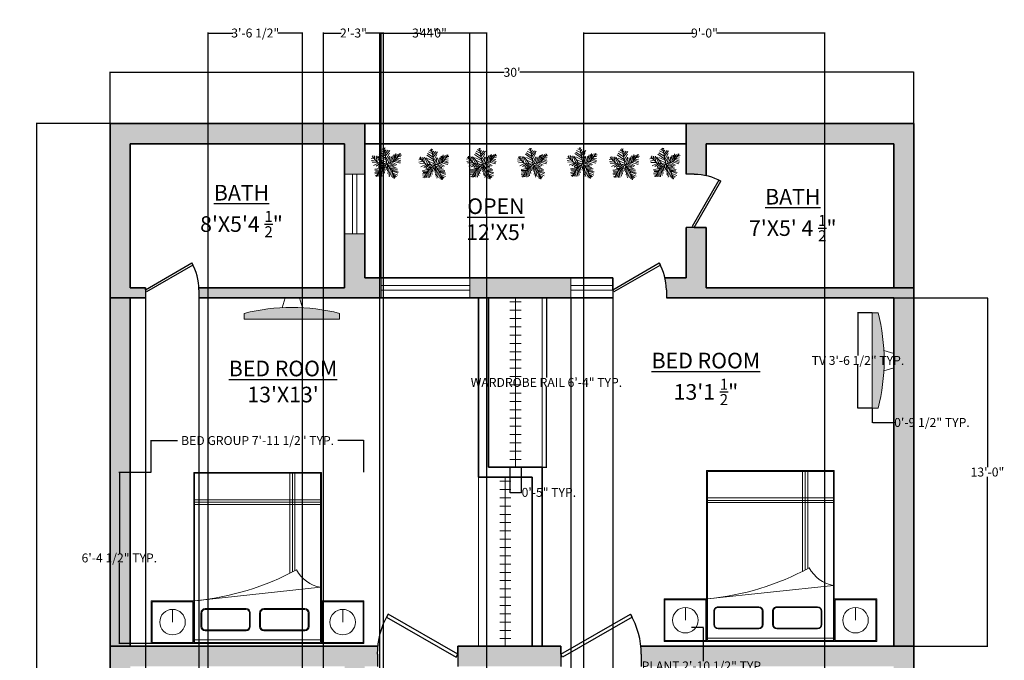
# Model space of a CAD drawing. Units: inches. Extents: x -37 to 408, y -619 to 75.
# Tile 4 of 4: x -37 to 404, y -212 to 75. Entities that reach past the tile are written whole.
import ezdxf

# ---------------------------------------------------------------- set-up
doc = ezdxf.new("R2010")
doc.units = ezdxf.units.IN
doc.header["$MEASUREMENT"] = 0
for name, color, linetype, lineweight in [('A-ANNO-DIMS', 2, 'Continuous', 18), ('A-AREA-IDEN', 7, 'Continuous', 25), ('A-DOOR', 4, 'Continuous', 25), ('A-EQPM', 9, 'Continuous', 18), ('A-FLOR-CASE', 8, 'Continuous', 18), ('A-FURN', 8, 'Continuous', 18), ('A-GLAZ', 4, 'Continuous', 18), ('A-WALL', 7, 'Continuous', 35), ('A-WALL-PATT', 16, 'Continuous', 13), ('tree', 3, 'Continuous', 13)]:
    doc.layers.add(name, color=color, linetype=linetype, lineweight=lineweight)
doc.styles.get("Standard").update_dxf_attribs({"font": 'arial.ttf'})
doc.dimstyles.get("Standard").update_dxf_attribs({"dimtxt": 4, "dimasz": 0.18, "dimexe": 0.18, "dimexo": 0.0625, "dimgap": 0.09, "dimtad": 0, "dimtih": 1, "dimtoh": 1, "dimdec": 1, "dimzin": 0, "dimdsep": 46, "dimlunit": 4, "dimtxsty": 'Standard', "dimcen": 0.09, "dimadec": 0, "dimazin": 0, "dimtfac": 1, "dimtdec": 1, "dimtofl": 0, "dimtmove": 0, "dimatfit": 3, "dimfxl": 1, "dimtolj": 1, "dimtzin": 0, "dimarcsym": 0})

# ---------------------------------------------------------------- blocks, each defined once
blk = doc.blocks.new('*U2')
for p, q in [((0, 0), (0, -6)), ((40, 0), (40, -6))]:
    blk.add_line(p, q)
blk.add_lwpolyline([(0, 0), (34.64, 20), (35.52, 18.48), (0.87, -1.52)], close=True)
blk.add_arc((0, 0), 40, 0, 30)
blk = doc.blocks.new('A$C0EA4476A')
at = {"linetype": 'ByBlock', "lineweight": -2}
for p, q in [((0, 2.008), (0, 1.508)), ((0.5, 2.008), (0, 2.008)), ((0.01, 1.998), (0.01, 1.518)), ((0.49, 1.998), (0.01, 1.998)), ((0.49, 1.518), (0.49, 1.998)), ((0.5, 2.008), (2, 2.008)), ((0.5, 0), (0.5, 2.008)), ((0.5, 1.508), (0.5, 2.008)), ((0.51, 1.998), (1.99, 1.998)), ((0.51, 0.01), (0.51, 1.998)), ((0.51, 1.968), (1.99, 1.968)), ((1.99, 1.998), (1.99, 0.01)), ((2, 2.008), (2, 0)), ((2, 2.008), (2.5, 2.008)), ((2, 1.508), (2, 2.008)), ((2.01, 1.998), (2.49, 1.998)), ((2.01, 1.518), (2.01, 1.998)), ((2.49, 1.998), (2.49, 1.518)), ((2.5, 2.008), (2.5, 1.508)), ((0.696, 1.86), (1.176, 1.86)), ((1.386, 1.86), (1.866, 1.86)), ((0.25, 1.758), (0.25, 1.608)), ((0.646, 1.65), (0.646, 1.81)), ((0.656, 1.65), (0.656, 1.81)), ((0.696, 1.85), (1.176, 1.85)), ((1.216, 1.81), (1.216, 1.65)), ((1.226, 1.81), (1.226, 1.65)), ((1.336, 1.65), (1.336, 1.81)), ((1.346, 1.65), (1.346, 1.81)), ((1.386, 1.85), (1.866, 1.85)), ((1.906, 1.81), (1.906, 1.65)), ((1.916, 1.81), (1.916, 1.65)), ((2.25, 1.758), (2.25, 1.608)), ((0, 1.508), (0.5, 1.508)), ((0.01, 1.518), (0.49, 1.518)), ((1.99, 1.508), (0.51, 1.349)), ((1.176, 1.61), (0.696, 1.61)), ((1.176, 1.6), (0.696, 1.6)), ((1.866, 1.61), (1.386, 1.61)), ((1.866, 1.6), (1.386, 1.6)), ((2.5, 1.508), (2, 1.508)), ((2.49, 1.518), (2.01, 1.518)), ((0.842, 1.169), (0.842, 0.01)), ((0.872, 1.184), (0.872, 0.01)), ((0.812, 1.153), (0.812, 0.01)), ((0.51, 0.377), (1.99, 0.377)), ((0.51, 0.35), (1.99, 0.35)), ((0.51, 0.322), (1.99, 0.322)), ((1.99, 0.01), (0.51, 0.01)), ((2, 0), (0.5, 0))]:
    blk.add_line(p, q, dxfattribs=at)
for centre in [(0.25, 1.758), (2.25, 1.758)]:
    blk.add_circle(centre, 0.15, dxfattribs=at)
for centre, radius, start, end in [((0.696, 1.81), 0.05, 90, 180), ((1.176, 1.81), 0.05, 0, 90), ((1.386, 1.81), 0.05, 90, 180), ((1.866, 1.81), 0.05, 0, 90), ((0.696, 1.81), 0.04, 90, 180), ((1.176, 1.81), 0.04, 0, 90), ((1.386, 1.81), 0.04, 90, 180), ((1.866, 1.81), 0.04, 0, 90), ((0.696, 1.65), 0.05, 180, 270), ((0.696, 1.65), 0.04, 180, 270), ((1.176, 1.65), 0.04, 270, 0), ((1.176, 1.65), 0.05, 270, 0), ((1.386, 1.65), 0.05, 180, 270), ((1.386, 1.65), 0.04, 180, 270), ((1.866, 1.65), 0.05, 270, 0), ((1.866, 1.65), 0.04, 270, 0), ((2.293, -1.636), 3.158, 95.5104, 118.3399), ((0.44, 0.952), 0.403, 28.4688, 79.9557)]:
    blk.add_arc(centre, radius, start, end, dxfattribs=at)
blk = doc.blocks.new('A$C1A706E3E')
blk.add_blockref('A$C0EA4476A', (0, 0))
blk = doc.blocks.new('Trees - Imperial')
for p, q in [((-3.665, 19.273), (-27.574, 35.527)), ((-5.114, 28.097), (-24.676, 40.636)), ((-7.288, 39.707), (-21.778, 46.673)), ((-8.737, 47.138), (-17.069, 52.711)), ((-10.186, 53.64), (-13.084, 55.962)), ((0, 0), (-10.5, 57)), ((-9.099, 51.782), (-6.563, 55.962)), ((-7.65, 43.423), (-2.578, 49.46)), ((-5.839, 35.992), (4.667, 48.067)), ((-5.114, 27.632), (10.463, 46.673)), ((-2.941, 16.486), (8.652, 37.85)), ((27, 9), (48, 36)), ((27.127, 9.056), (31.112, 35.992)), ((44.153, 36.456), (45.239, 32.741)), ((-47.498, 19.737), (-55.83, 18.344)), ((-40.615, 13.7), (-55.105, 10.913)), ((-31.5, 4.5), (-52.5, 25.5)), ((-33.37, 6.269), (-52.207, 5.34)), ((-48.585, 21.131), (-49.309, 29.026)), ((-28.299, 3.483), (-47.86, -5.805)), ((-43.513, 28.561), (-42.427, 15.558)), ((-38.442, 26.239), (-34.819, 7.663)), ((-21.416, 3.018), (-38.079, -8.128)), ((-35.544, 28.097), (-24.314, 3.947)), ((0, 0), (-31.5, 4.5)), ((-14.533, 2.09), (-30.834, 25.31)), ((-15.982, 2.09), (-30.11, -9.521)), ((-24.314, 23.917), (-2.941, 13.7)), ((0, 0), (-22.5, -19.5)), ((-6.563, 1.161), (-21.416, -8.128)), ((-20.691, 13.7), (-1.129, 4.876)), ((-1.129, 6.734), (9.014, 26.704)), ((0, 0), (27, 9)), ((0, 0), (18, -22.5)), ((3.942, 1.625), (11.187, 24.381)), ((6.478, 1.625), (26.04, -8.592)), ((10.101, 3.483), (17.708, 26.239)), ((11.187, 3.483), (30.749, -5.805)), ((16.259, 5.805), (23.142, 31.348)), ((18.07, 5.805), (35.096, -3.483)), ((22.055, 7.198), (27.489, 32.277)), ((24.229, 7.663), (46.688, 1.625)), ((29.662, 12.307), (48.137, 6.269)), ((31.836, 30.883), (32.561, 16.486)), ((33.285, 16.486), (48.862, 10.913)), ((35.096, 32.741), (37.27, 22.524)), ((36.183, 19.737), (48.137, 17.88)), ((38.719, 34.134), (41.979, 28.561)), ((40.53, 25.775), (48.862, 24.846)), ((43.791, 29.954), (51.036, 30.883)), ((-17.431, -15.094), (-42.789, -18.809)), ((-28.299, -29.026), (-42.789, -31.348)), ((-24.314, -21.596), (-42.427, -22.06)), ((-30.834, -34.135), (-42.427, -35.528)), ((-26.849, -26.24), (-40.253, -25.775)), ((-22.5, -19.5), (-37.5, -45)), ((-15.257, -12.772), (-30.11, -12.772)), ((-29.023, -30.884), (-27.936, -43.887)), ((-25.038, -23.918), (-22.865, -45.281)), ((-20.691, -18.345), (-17.793, -44.352)), ((-6.563, -5.805), (-19.967, -9.985)), ((-17.069, -15.094), (-12.721, -40.172)), ((-13.446, -11.378), (-8.737, -32.741)), ((-9.461, -8.592), (-6.201, -23.453)), ((-4.752, -3.483), (-3.665, -14.629)), ((2.493, -3.019), (-1.491, -20.202)), ((1.769, -2.555), (24.229, -9.521)), ((5.029, -6.27), (2.131, -25.775)), ((9.014, -11.378), (3.58, -35.992)), ((14.085, -16.951), (6.478, -40.172)), ((7.565, -9.056), (32.198, -14.629)), ((18.07, -22.524), (8.289, -45.745)), ((12.274, -15.094), (36.907, -18.809)), ((20.244, -30.419), (15.897, -44.816)), ((16.259, -19.738), (36.183, -22.989)), ((18, -22.5), (27, -52.5)), ((18.433, -22.524), (40.53, -29.026)), ((19.157, -25.311), (38.719, -33.206)), ((21.331, -32.741), (39.081, -40.636)), ((-34.457, -39.708), (-40.978, -42.494)), ((-32.646, -36.921), (-31.921, -44.352)), ((22.78, -37.85), (19.519, -48.532)), ((22.78, -38.314), (34.372, -44.816)), ((24.591, -45.745), (23.142, -50.854)), ((24.591, -43.423), (30.749, -47.603)), ((26.764, -49.925), (28.213, -50.854))]:
    blk.add_line(p, q)
blk = doc.blocks.new('*D11')
at = {"layer": 'A-ANNO-DIMS', "color": 0, "lineweight": -2, "transparency": 16777216}
for p, q in [((3.58, 28.69), (3.58, 51.78)), ((3.76, 51.6), (180.1, 51.6)), ((363.4, 51.6), (187.06, 51.6)), ((363.58, 28.69), (363.58, 51.78))]:
    blk.add_line(p, q, dxfattribs=at)
at = {"layer": 'A-ANNO-DIMS', "color": 0, "transparency": 16777216}
for points in [[(3.76, 51.63), (3.76, 51.57), (3.58, 51.6)], [(363.4, 51.63), (363.4, 51.57), (363.58, 51.6)]]:
    blk.add_solid(points, dxfattribs=at)
at = {"layer": 'Defpoints', "color": 0, "transparency": 16777216}
for p in [(363.58, 51.6), (3.58, 28.62), (363.58, 28.62)]:
    blk.add_point(p, dxfattribs=at)
at = {"layer": 'A-ANNO-DIMS', "color": 0, "transparency": 16777216, "insert": (183.58, 51.6), "char_height": 4, "attachment_point": 5}
blk.add_mtext("\\A1;30'", dxfattribs=at)
blk = doc.blocks.new('TV-WALL-MOUNT')
h = blk.add_hatch(color=256)
h.dxf.hatch_style = 1
h.set_gradient(color1=(255, 255, 255), color2=(0, 255, 255), tint=1, name='CYLINDER')
h.paths.add_polyline_path([(21.48, 5.31), (21.22, 5.31, 0.06152), (0, 2.65), (0, 0), (21.35, 0), (42.7, 0), (42.7, 2.65, 0.06152)])
for p, q in [((18.26, 9.61), (16.92, 5.19)), ((24.71, 9.61), (26.04, 5.19)), ((23.28, 5.31), (19.68, 5.31)), ((0, 2.65), (0, 0)), ((0, 0), (21.35, 0)), ((42.7, 0), (21.35, 0)), ((42.7, 2.65), (42.7, 0))]:
    blk.add_line(p, q)
blk.add_arc((21.35, -81.94), 87.25, 75.8341, 104.1659)
blk = doc.blocks.new('WARDROBE-HANGING-RAIL')
for p, q in [((2.46, 0), (2.46, 75.75)), ((0, 73.9), (5, 73.9)), ((0, 70.19), (5, 70.19)), ((0, 66.48), (5, 66.48)), ((0, 62.77), (5, 62.77)), ((0, 59.05), (5, 59.05)), ((0, 55.34), (5, 55.34)), ((0, 51.63), (5, 51.63)), ((0, 47.92), (5, 47.92)), ((0, 44.21), (5, 44.21)), ((0, 40.5), (5, 40.5)), ((0, 36.79), (5, 36.79)), ((0, 33.08), (5, 33.08)), ((0, 29.37), (5, 29.37)), ((0, 25.65), (5, 25.65)), ((0, 21.94), (5, 21.94)), ((0, 18.23), (5, 18.23)), ((0, 14.52), (5, 14.52)), ((0, 10.81), (5, 10.81)), ((0, 7.1), (5, 7.1)), ((0, 3.39), (5, 3.39))]:
    blk.add_line(p, q)
blk = doc.blocks.new('*D14')
at = {"layer": 'A-ANNO-DIMS', "color": 0, "lineweight": -2, "transparency": 16777216}
for p, q in [((264.05, -196.9), (269.35, -196.9)), ((269.17, -197.08), (269.17, -212.04)), ((269.17, -231.31), (269.17, -216.35)), ((264.05, -231.49), (269.35, -231.49))]:
    blk.add_line(p, q, dxfattribs=at)
at = {"layer": 'A-ANNO-DIMS', "color": 0, "transparency": 16777216}
for points in [[(269.14, -197.08), (269.2, -197.08), (269.17, -196.9)], [(269.14, -231.31), (269.2, -231.31), (269.17, -231.49)]]:
    blk.add_solid(points, dxfattribs=at)
at = {"layer": 'Defpoints', "color": 0, "transparency": 16777216}
for p in [(263.98, -196.9), (269.17, -196.9), (263.98, -231.49)]:
    blk.add_point(p, dxfattribs=at)
at = {"layer": 'A-ANNO-DIMS', "color": 0, "transparency": 16777216, "insert": (269.17, -214.2), "char_height": 4, "attachment_point": 5}
blk.add_mtext('\\A1;PLANT 2\'-10 1/2" TYP.', dxfattribs=at)
blk = doc.blocks.new('*D16')
at = {"layer": 'A-ANNO-DIMS', "color": 0, "lineweight": -2, "transparency": 16777216}
for p, q in [((344.9, -56.07), (338.38, -56.07)), ((338.56, -56.25), (338.56, -75.26)), ((338.56, -98.59), (338.56, -79.58)), ((344.9, -98.77), (338.38, -98.77))]:
    blk.add_line(p, q, dxfattribs=at)
at = {"layer": 'A-ANNO-DIMS', "color": 0, "transparency": 16777216}
for points in [[(338.53, -56.25), (338.59, -56.25), (338.56, -56.07)], [(338.53, -98.59), (338.59, -98.59), (338.56, -98.77)]]:
    blk.add_solid(points, dxfattribs=at)
at = {"layer": 'Defpoints', "color": 0, "transparency": 16777216}
for p in [(344.97, -56.07), (338.56, -98.77), (344.97, -98.77)]:
    blk.add_point(p, dxfattribs=at)
at = {"layer": 'A-ANNO-DIMS', "color": 0, "transparency": 16777216, "insert": (338.56, -77.42), "char_height": 4, "attachment_point": 5}
blk.add_mtext('\\A1;TV 3\'-6 1/2" TYP.', dxfattribs=at)
blk = doc.blocks.new('*D17')
at = {"layer": 'A-ANNO-DIMS', "color": 0, "lineweight": -2, "transparency": 16777216}
for p, q in [((344.97, -98.84), (344.97, -105.36)), ((354.58, -98.84), (354.58, -105.36)), ((345.15, -105.18), (354.4, -105.18)), ((354.58, -105.18), (354.76, -105.18))]:
    blk.add_line(p, q, dxfattribs=at)
at = {"layer": 'A-ANNO-DIMS', "color": 0, "transparency": 16777216}
for points in [[(345.15, -105.15), (345.15, -105.21), (344.97, -105.18)], [(354.4, -105.15), (354.4, -105.21), (354.58, -105.18)]]:
    blk.add_solid(points, dxfattribs=at)
at = {"layer": 'Defpoints', "color": 0, "transparency": 16777216}
for p in [(344.97, -98.77), (354.58, -98.77), (354.58, -105.18)]:
    blk.add_point(p, dxfattribs=at)
at = {"layer": 'A-ANNO-DIMS', "color": 0, "transparency": 16777216, "insert": (371.7, -105.18), "char_height": 4, "attachment_point": 5}
blk.add_mtext('\\A1;0\'-9 1/2" TYP.', dxfattribs=at)
blk = doc.blocks.new('*D18')
at = {"layer": 'A-ANNO-DIMS', "color": 0, "lineweight": -2, "transparency": 16777216}
for p, q in [((21.97, -127.51), (21.97, -113.1)), ((22.15, -113.28), (33.67, -113.28)), ((117.09, -113.28), (105.57, -113.28)), ((117.27, -127.51), (117.27, -113.1))]:
    blk.add_line(p, q, dxfattribs=at)
at = {"layer": 'A-ANNO-DIMS', "color": 0, "transparency": 16777216}
for points in [[(22.15, -113.25), (22.15, -113.31), (21.97, -113.28)], [(117.09, -113.25), (117.09, -113.31), (117.27, -113.28)]]:
    blk.add_solid(points, dxfattribs=at)
at = {"layer": 'Defpoints', "color": 0, "transparency": 16777216}
for p in [(21.97, -113.28), (21.97, -127.57), (117.27, -127.57)]:
    blk.add_point(p, dxfattribs=at)
at = {"layer": 'A-ANNO-DIMS', "color": 0, "transparency": 16777216, "insert": (69.62, -113.28), "char_height": 4, "attachment_point": 5}
blk.add_mtext('\\A1;BED GROUP 7\'-11 1/2" TYP.', dxfattribs=at)
blk = doc.blocks.new('*D19')
at = {"layer": 'A-ANNO-DIMS', "color": 0, "lineweight": -2, "transparency": 16777216}
for p, q in [((21.91, -127.57), (7.5, -127.57)), ((7.68, -127.75), (7.68, -163.69)), ((7.68, -203.93), (7.68, -168)), ((21.91, -204.11), (7.5, -204.11))]:
    blk.add_line(p, q, dxfattribs=at)
at = {"layer": 'A-ANNO-DIMS', "color": 0, "transparency": 16777216}
for points in [[(7.65, -127.75), (7.71, -127.75), (7.68, -127.57)], [(7.65, -203.93), (7.71, -203.93), (7.68, -204.11)]]:
    blk.add_solid(points, dxfattribs=at)
at = {"layer": 'Defpoints', "color": 0, "transparency": 16777216}
for p in [(21.97, -127.57), (7.68, -204.11), (21.97, -204.11)]:
    blk.add_point(p, dxfattribs=at)
at = {"layer": 'A-ANNO-DIMS', "color": 0, "transparency": 16777216, "insert": (7.68, -165.84), "char_height": 4, "attachment_point": 5}
blk.add_mtext('\\A1;6\'-4 1/2" TYP.', dxfattribs=at)
blk = doc.blocks.new('*D20')
at = {"layer": 'A-ANNO-DIMS', "color": 0, "lineweight": -2, "transparency": 16777216}
for p, q in [((187.69, -49.38), (199.17, -49.38)), ((198.99, -49.56), (198.99, -85.09)), ((198.99, -124.95), (198.99, -89.41)), ((187.69, -125.13), (199.17, -125.13))]:
    blk.add_line(p, q, dxfattribs=at)
at = {"layer": 'A-ANNO-DIMS', "color": 0, "transparency": 16777216}
for points in [[(198.96, -49.56), (199.02, -49.56), (198.99, -49.38)], [(198.96, -124.95), (199.02, -124.95), (198.99, -125.13)]]:
    blk.add_solid(points, dxfattribs=at)
at = {"layer": 'Defpoints', "color": 0, "transparency": 16777216}
for p in [(187.63, -49.38), (198.99, -49.38), (187.63, -125.13)]:
    blk.add_point(p, dxfattribs=at)
at = {"layer": 'A-ANNO-DIMS', "color": 0, "transparency": 16777216, "insert": (198.99, -87.25), "char_height": 4, "attachment_point": 5}
blk.add_mtext('\\A1;WARDROBE RAIL 6\'-4" TYP.', dxfattribs=at)
blk = doc.blocks.new('*D21')
at = {"layer": 'A-ANNO-DIMS', "color": 0, "lineweight": -2, "transparency": 16777216}
for p, q in [((182.62, -125.19), (182.62, -136.67)), ((187.63, -125.19), (187.63, -136.67)), ((182.8, -136.49), (187.45, -136.49)), ((187.63, -136.49), (187.81, -136.49))]:
    blk.add_line(p, q, dxfattribs=at)
at = {"layer": 'A-ANNO-DIMS', "color": 0, "transparency": 16777216}
for points in [[(182.8, -136.46), (182.8, -136.52), (182.62, -136.49)], [(187.45, -136.46), (187.45, -136.52), (187.63, -136.49)]]:
    blk.add_solid(points, dxfattribs=at)
at = {"layer": 'Defpoints', "color": 0, "transparency": 16777216}
for p in [(182.62, -125.13), (187.63, -125.13), (187.63, -136.49)]:
    blk.add_point(p, dxfattribs=at)
at = {"layer": 'A-ANNO-DIMS', "color": 0, "transparency": 16777216, "insert": (200.09, -136.49), "char_height": 4, "attachment_point": 5}
blk.add_mtext('\\A1;0\'-5" TYP.', dxfattribs=at)
blk = doc.blocks.new('*D28')
at = {"layer": 'A-ANNO-DIMS', "color": 0, "lineweight": -2, "transparency": 16777216}
for p, q in [((3.52, 28.62), (-29.6, 28.62)), ((-29.42, 28.44), (-29.42, -273.74)), ((-29.42, -580.2), (-29.42, -278.01)), ((3.52, -580.38), (-29.6, -580.38))]:
    blk.add_line(p, q, dxfattribs=at)
at = {"layer": 'A-ANNO-DIMS', "color": 0, "transparency": 16777216}
for points in [[(-29.45, 28.44), (-29.39, 28.44), (-29.42, 28.62)], [(-29.45, -580.2), (-29.39, -580.2), (-29.42, -580.38)]]:
    blk.add_solid(points, dxfattribs=at)
at = {"layer": 'Defpoints', "color": 0, "transparency": 16777216}
for p in [(-29.42, 28.62), (3.58, 28.62), (3.58, -580.38)]:
    blk.add_point(p, dxfattribs=at)
at = {"layer": 'A-ANNO-DIMS', "color": 0, "transparency": 16777216, "insert": (-29.42, -275.88), "char_height": 4, "attachment_point": 5}
blk.add_mtext('\\A1;50\'-9"', dxfattribs=at)
blk = doc.blocks.new('*D29')
at = {"layer": 'A-ANNO-DIMS', "color": 0, "lineweight": -2, "transparency": 16777216}
for p, q in [((354.64, -49.38), (396.76, -49.38)), ((396.58, -49.56), (396.58, -125.24)), ((396.58, -205.2), (396.58, -129.51)), ((354.64, -205.38), (396.76, -205.38))]:
    blk.add_line(p, q, dxfattribs=at)
at = {"layer": 'A-ANNO-DIMS', "color": 0, "transparency": 16777216}
for points in [[(396.55, -49.56), (396.61, -49.56), (396.58, -49.38)], [(396.55, -205.2), (396.61, -205.2), (396.58, -205.38)]]:
    blk.add_solid(points, dxfattribs=at)
at = {"layer": 'Defpoints', "color": 0, "transparency": 16777216}
for p in [(354.58, -49.38), (396.58, -49.38), (354.58, -205.38)]:
    blk.add_point(p, dxfattribs=at)
at = {"layer": 'A-ANNO-DIMS', "color": 0, "transparency": 16777216, "insert": (396.58, -127.38), "char_height": 4, "attachment_point": 5}
blk.add_mtext('\\A1;13\'-0"', dxfattribs=at)
blk = doc.blocks.new('*D34')
at = {"layer": 'A-ANNO-DIMS', "color": 0, "lineweight": -2, "transparency": 16777216}
for p, q in [((124.36, -346.31), (124.36, 69.37)), ((124.54, 69.19), (142.88, 69.19)), ((172.18, 69.19), (153.85, 69.19)), ((172.36, -346.31), (172.36, 69.37))]:
    blk.add_line(p, q, dxfattribs=at)
at = {"layer": 'A-ANNO-DIMS', "color": 0, "transparency": 16777216}
for points in [[(124.54, 69.22), (124.54, 69.16), (124.36, 69.19)], [(172.18, 69.22), (172.18, 69.16), (172.36, 69.19)]]:
    blk.add_solid(points, dxfattribs=at)
at = {"layer": 'Defpoints', "color": 0, "transparency": 16777216}
for p in [(172.36, 69.19), (124.36, -346.38), (172.36, -346.38)]:
    blk.add_point(p, dxfattribs=at)
at = {"layer": 'A-ANNO-DIMS', "color": 0, "transparency": 16777216, "insert": (148.36, 69.19), "char_height": 4, "attachment_point": 5}
blk.add_mtext('\\A1;4\'-0"', dxfattribs=at)
blk = doc.blocks.new('*D39')
at = {"layer": 'A-ANNO-DIMS', "color": 0, "lineweight": -2, "transparency": 16777216}
for p, q in [((19.34, -49.44), (19.34, -613.56)), ((43.34, -49.44), (43.34, -613.56)), ((19.52, -613.38), (25.9, -613.38)), ((43.16, -613.38), (36.78, -613.38))]:
    blk.add_line(p, q, dxfattribs=at)
at = {"layer": 'A-ANNO-DIMS', "color": 0, "transparency": 16777216}
for points in [[(19.52, -613.35), (19.52, -613.41), (19.34, -613.38)], [(43.16, -613.35), (43.16, -613.41), (43.34, -613.38)]]:
    blk.add_solid(points, dxfattribs=at)
at = {"layer": 'Defpoints', "color": 0, "transparency": 16777216}
for p in [(19.34, -49.38), (43.34, -49.38), (43.34, -613.38)]:
    blk.add_point(p, dxfattribs=at)
at = {"layer": 'A-ANNO-DIMS', "color": 0, "transparency": 16777216, "insert": (31.34, -613.38), "char_height": 4, "attachment_point": 5}
blk.add_mtext('\\A1;2\'-0"', dxfattribs=at)
blk = doc.blocks.new('*D43')
at = {"layer": 'A-ANNO-DIMS', "color": 0, "lineweight": -2, "transparency": 16777216}
for p, q in [((47.42, -343.92), (47.42, 69.37)), ((47.6, 69.19), (58.49, 69.19)), ((89.51, 69.19), (78.62, 69.19)), ((89.69, -343.92), (89.69, 69.37))]:
    blk.add_line(p, q, dxfattribs=at)
at = {"layer": 'A-ANNO-DIMS', "color": 0, "transparency": 16777216}
for points in [[(47.6, 69.22), (47.6, 69.16), (47.42, 69.19)], [(89.51, 69.22), (89.51, 69.16), (89.69, 69.19)]]:
    blk.add_solid(points, dxfattribs=at)
at = {"layer": 'Defpoints', "color": 0, "transparency": 16777216}
for p in [(89.69, 69.19), (47.42, -343.98), (89.69, -343.98)]:
    blk.add_point(p, dxfattribs=at)
at = {"layer": 'A-ANNO-DIMS', "color": 0, "transparency": 16777216, "insert": (68.55, 69.19), "char_height": 4, "attachment_point": 5}
blk.add_mtext('\\A1;3\'-6 1/2"', dxfattribs=at)
blk = doc.blocks.new('*D47')
at = {"layer": 'A-ANNO-DIMS', "color": 0, "lineweight": -2, "transparency": 16777216}
for p, q in [((124.92, -40.31), (124.92, 69.37)), ((125.1, 69.19), (139.43, 69.19)), ((164.58, 69.19), (150.24, 69.19)), ((164.76, -40.31), (164.76, 69.37))]:
    blk.add_line(p, q, dxfattribs=at)
at = {"layer": 'A-ANNO-DIMS', "color": 0, "transparency": 16777216}
for points in [[(125.1, 69.22), (125.1, 69.16), (124.92, 69.19)], [(164.58, 69.22), (164.58, 69.16), (164.76, 69.19)]]:
    blk.add_solid(points, dxfattribs=at)
at = {"layer": 'Defpoints', "color": 0, "transparency": 16777216}
for p in [(164.76, 69.19), (124.92, -40.38), (164.76, -40.38)]:
    blk.add_point(p, dxfattribs=at)
at = {"layer": 'A-ANNO-DIMS', "color": 0, "transparency": 16777216, "insert": (144.84, 69.19), "char_height": 4, "attachment_point": 5}
blk.add_mtext('\\A1;3\'-4"', dxfattribs=at)
blk = doc.blocks.new('*D48')
at = {"layer": 'A-ANNO-DIMS', "color": 0, "lineweight": -2, "transparency": 16777216}
for p, q in [((209.99, -49.44), (209.99, -613.56)), ((228.72, -49.44), (228.72, -613.56)), ((210.17, -613.38), (228.54, -613.38)), ((228.72, -613.38), (228.9, -613.38))]:
    blk.add_line(p, q, dxfattribs=at)
at = {"layer": 'A-ANNO-DIMS', "color": 0, "transparency": 16777216}
for points in [[(210.17, -613.35), (210.17, -613.41), (209.99, -613.38)], [(228.54, -613.35), (228.54, -613.41), (228.72, -613.38)]]:
    blk.add_solid(points, dxfattribs=at)
at = {"layer": 'Defpoints', "color": 0, "transparency": 16777216}
for p in [(209.99, -49.38), (228.72, -49.38), (228.72, -613.38)]:
    blk.add_point(p, dxfattribs=at)
at = {"layer": 'A-ANNO-DIMS', "color": 0, "transparency": 16777216, "insert": (238.78, -613.38), "char_height": 4, "attachment_point": 5}
blk.add_mtext('\\A1;1\'-6 1/2"', dxfattribs=at)
blk = doc.blocks.new('*D50')
at = {"layer": 'A-ANNO-DIMS', "color": 0, "lineweight": -2, "transparency": 16777216}
for p, q in [((215.83, -476.93), (215.83, 69.37)), ((216.01, 69.19), (264.38, 69.19)), ((323.57, 69.19), (275.2, 69.19)), ((323.75, -477.22), (323.75, 69.37))]:
    blk.add_line(p, q, dxfattribs=at)
at = {"layer": 'A-ANNO-DIMS', "color": 0, "transparency": 16777216}
for points in [[(216.01, 69.22), (216.01, 69.16), (215.83, 69.19)], [(323.57, 69.22), (323.57, 69.16), (323.75, 69.19)]]:
    blk.add_solid(points, dxfattribs=at)
at = {"layer": 'Defpoints', "color": 0, "transparency": 16777216}
for p in [(323.75, 69.19), (215.83, -476.99), (323.75, -477.28)]:
    blk.add_point(p, dxfattribs=at)
at = {"layer": 'A-ANNO-DIMS', "color": 0, "transparency": 16777216, "insert": (269.79, 69.19), "char_height": 4, "attachment_point": 5}
blk.add_mtext('\\A1;9\'-0"', dxfattribs=at)
blk = doc.blocks.new('*D53')
at = {"layer": 'A-ANNO-DIMS', "color": 0, "lineweight": -2, "transparency": 16777216}
for p, q in [((99.07, -267.5), (99.07, 69.37)), ((99.25, 69.19), (107.12, 69.19)), ((125.88, 69.19), (118, 69.19)), ((126.06, -267.5), (126.06, 69.37))]:
    blk.add_line(p, q, dxfattribs=at)
at = {"layer": 'A-ANNO-DIMS', "color": 0, "transparency": 16777216}
for points in [[(99.25, 69.22), (99.25, 69.16), (99.07, 69.19)], [(125.88, 69.22), (125.88, 69.16), (126.06, 69.19)]]:
    blk.add_solid(points, dxfattribs=at)
at = {"layer": 'Defpoints', "color": 0, "transparency": 16777216}
for p in [(126.06, 69.19), (99.07, -267.56), (126.06, -267.56)]:
    blk.add_point(p, dxfattribs=at)
at = {"layer": 'A-ANNO-DIMS', "color": 0, "transparency": 16777216, "insert": (112.56, 69.19), "char_height": 4, "attachment_point": 5}
blk.add_mtext('\\A1;2\'-3"', dxfattribs=at)

msp = doc.modelspace()

# ---------------------------------------------------------------- hatches: boundary and pattern name
at = {"layer": 'A-WALL-PATT'}
h = msp.add_hatch(color=256, dxfattribs=at)
h.dxf.hatch_style = 1
h.paths.add_polyline_path([(117.58, 28.62), (3.58, 28.62), (3.58, -49.38), (19.34, -49.38), (19.34, -45.78), (19.34, -44.88), (12.58, -44.88), (12.58, 19.62), (108.58, 19.62), (108.58, 5.94), (117.58, 5.94), (117.58, 19.62)])
h.paths.add_polyline_path([(363.58, 28.62), (261.58, 28.62), (261.58, 19.62), (261.58, 6.04), (265.18, 6.04, -0.056797), (270.58, 5.42), (270.58, 19.62), (354.58, 19.62), (354.58, -44.88), (363.58, -44.88)])
h.paths.add_polyline_path([(124.92, -40.38), (117.58, -40.38), (117.58, -20.71), (108.58, -20.71), (108.58, -44.88), (43.33, -44.88, -0.009377), (43.34, -45.78), (43.34, -49.38), (124.92, -49.38)])
h.paths.add_polyline_path([(209.99, -40.38), (164.76, -40.38), (164.76, -49.38), (209.99, -49.38)])
h.paths.add_polyline_path([(270.58, -17.96), (265.18, -17.96), (261.58, -17.96), (261.58, -40.38), (252.1, -40.38, -0.056797), (252.72, -45.78), (252.72, -49.38), (354.58, -49.38), (354.58, -205.38), (363.58, -205.38), (363.58, -44.88), (354.58, -44.88), (270.58, -44.88)])
h.paths.add_polyline_path([(12.58, -49.38), (3.58, -49.38), (3.58, -205.38), (12.58, -205.38)])
h.paths.add_polyline_path([(205.47, -208.98), (205.47, -205.38), (159.34, -205.38), (159.34, -208.98), (159.34, -214.38), (205.47, -214.38)])
h = msp.add_hatch(color=256, dxfattribs=at)
h.dxf.hatch_style = 1
h.paths.add_polyline_path([(123.52, -205.38), (3.58, -205.38), (3.58, -355.38), (27.35, -355.38), (27.35, -346.38), (12.58, -346.38), (12.58, -214.38), (123.34, -214.38), (123.34, -208.98, -0.025047)])
h.paths.add_polyline_path([(117.58, -214.38), (108.58, -214.38), (108.58, -221.31), (112.18, -221.31), (117.58, -221.31)], flags=17)
h.paths.add_polyline_path([(124.36, -346.38), (86.98, -346.38), (86.98, -355.38), (124.36, -355.38), (124.36, -351.78)])
h.paths.add_polyline_path([(222.97, -346.38), (172.36, -346.38), (172.36, -351.78), (172.36, -355.38), (180.58, -355.38), (180.58, -364.83), (185.98, -364.83), (189.58, -364.83), (189.58, -355.38), (222.97, -355.38)])
h.paths.add_polyline_path([(363.58, -205.38), (241.29, -205.38, -0.025047), (241.47, -208.98), (241.47, -214.38), (354.58, -214.38), (354.58, -346.38), (317.68, -346.38), (317.68, -355.38), (363.58, -355.38)])

# ---------------------------------------------------------------- linework, layer by layer
at = {"layer": 'A-FLOR-CASE'}
for p, q in [((197.08, -125.13), (197.08, -49.38)), ((168.58, -129.63), (168.58, -205.38))]:
    msp.add_line(p, q, dxfattribs=at)
at = {"layer": 'A-GLAZ'}
for p, q in [((108.58, 5.94), (117.58, 5.94)), ((112.08, 5.94), (112.08, -20.71)), ((114.08, 5.94), (114.08, -20.71)), ((108.58, -20.71), (117.58, -20.71)), ((124.92, -40.38), (124.92, -49.38)), ((124.92, -43.88), (164.76, -43.88)), ((164.76, -49.38), (164.76, -40.38)), ((209.99, -40.38), (209.99, -49.38)), ((209.99, -43.88), (228.72, -43.88)), ((124.92, -45.88), (164.76, -45.88)), ((209.99, -45.88), (228.72, -45.88))]:
    msp.add_line(p, q, dxfattribs=at)
at = {"layer": 'A-WALL'}
for p, q in [((3.58, 28.62), (363.58, 28.62)), ((3.58, 28.62), (3.58, -580.38)), ((117.58, 19.62), (117.58, 28.62)), ((261.58, 19.62), (261.58, 28.62)), ((363.58, 28.62), (363.58, -580.38)), ((12.58, 19.62), (108.58, 19.62)), ((12.58, 19.62), (12.58, -44.88)), ((108.58, 19.62), (108.58, -44.88)), ((117.58, 19.62), (117.58, -40.38)), ((117.58, 19.62), (261.58, 19.62)), ((261.58, 19.62), (261.58, 6.04)), ((270.58, 19.62), (270.58, 5.42)), ((270.58, 19.62), (354.58, 19.62)), ((354.58, 19.62), (354.58, -44.88)), ((261.58, -17.96), (261.58, -40.38)), ((265.18, -17.96), (270.58, -17.96)), ((270.58, -17.96), (270.58, -44.88)), ((117.58, -40.38), (228.72, -40.38)), ((228.72, -45.78), (228.72, -40.38)), ((252.1, -40.38), (261.58, -40.38)), ((12.58, -44.88), (19.34, -44.88)), ((19.34, -45.78), (19.34, -44.88)), ((43.33, -44.88), (108.58, -44.88)), ((270.58, -44.88), (363.58, -44.88)), ((3.58, -49.38), (19.34, -49.38)), ((12.58, -49.38), (12.58, -205.38)), ((43.34, -49.38), (228.72, -49.38)), ((168.58, -49.38), (168.58, -129.63)), ((173.08, -49.38), (173.08, -125.13)), ((252.72, -49.38), (354.58, -49.38)), ((354.58, -49.38), (354.58, -205.38)), ((197.08, -125.13), (173.08, -125.13)), ((197.08, -125.13), (197.08, -205.38)), ((192.58, -129.63), (168.58, -129.63)), ((192.58, -129.63), (192.58, -205.38)), ((3.58, -205.38), (123.52, -205.38)), ((159.34, -208.98), (159.34, -205.38)), ((159.34, -205.38), (205.47, -205.38)), ((205.47, -208.98), (205.47, -205.38)), ((241.29, -205.38), (363.58, -205.38))]:
    msp.add_line(p, q, dxfattribs=at)

# ---------------------------------------------------------------- block references
at = {"layer": 'A-DOOR', "xscale": -0.6, "yscale": 0.6, "zscale": 0.6, "rotation": 270}
msp.add_blockref('*U2', (265.18, -17.96), dxfattribs=at)
at = {"layer": 'A-DOOR'}
for p, xscale, yscale, zscale in [((19.34, -45.78), 0.6, 0.6, 0.6), ((228.72, -45.78), 0.6, 0.6, 0.6), ((159.34, -208.98), -0.9, 0.9, 0.9), ((205.47, -208.98), 0.9, 0.9, 0.9)]:
    msp.add_blockref('*U2', p, dxfattribs=dict(at, xscale=xscale, yscale=yscale, zscale=zscale))
at = {"layer": 'A-EQPM'}
msp.add_blockref('TV-WALL-MOUNT', (63.65, -58.99), dxfattribs=at)
at = {"layer": 'A-EQPM', "rotation": 270}
msp.add_blockref('TV-WALL-MOUNT', (344.97, -56.07), dxfattribs=at)
at = {"layer": 'A-FLOR-CASE'}
for p in [(182.62, -125.13), (178.12, -205.38)]:
    msp.add_blockref('WARDROBE-HANGING-RAIL', p, dxfattribs=at)
at = {"layer": 'A-FURN', "xscale": 38.11722911383665, "yscale": 38.11722911383665, "zscale": 38.11722911383665, "rotation": 180}
for p in [(117.27, -127.57), (347.01, -126.72)]:
    msp.add_blockref('A$C1A706E3E', p, dxfattribs=at)
at = {"layer": 'tree', "xscale": 0.1267004668732905, "yscale": 0.1267004668732905, "zscale": 0.1267004668732905}
for p in [(127.54, 10.64), (215.26, 10.7), (252.43, 10.47), (148.86, 10.05), (170.31, 10.34), (193.08, 10.41), (234.2, 10.18)]:
    msp.add_blockref('Trees - Imperial', p, dxfattribs=at)

# ---------------------------------------------------------------- texts
at = {"layer": 'A-AREA-IDEN', "char_height": 7, "attachment_point": 1}
for s, insert in [('\\A1;\\pxqc;{\\fArial|b1|i0|c0|p34;\\LBATH\\P\\l8\'X5\'4 \\H0.7x;\\S1/2;\\H1.42857x;"}', (33.81, 1.2)), ('\\A1;\\pxqc;{\\fArial|b1|i0|c0|p34;\\LBATH\\l\\P7\'X5\' 4 \\H0.7x;\\S1/2;\\H1.42857x;"}', (280.78, -0.6)), ("\\A1;\\pxqc;{\\fArial|b1|i0|c0|p34;\\LOPEN\\P\\l12'X5'}", (147.79, -4.83)), ('\\A1;\\pxqc;{\\fArial|b1|i0|c0|p34;\\LBED ROOM\\l\\P13\'1 \\H0.7x;\\S1/2;\\H1.42857x;"}', (241.86, -73.96)), ("\\A1;\\pxqc;{\\fArial|b1|i0|c0|p34;\\LBED ROOM\\l\\P13'X13'}", (52.43, -77.51))]:
    msp.add_mtext_dynamic_manual_height_columns(s, width=57.1656, gutter_width=1, heights=[0], dxfattribs=dict(at, insert=insert))

# ---------------------------------------------------------------- dimensions: what is measured, and where the dimension line sits
at = {"layer": 'A-ANNO-DIMS'}
for base, p1, p2, override, picture, middle in [((89.69, 69.19), (47.42, -343.98), (89.69, -343.98), {"dimdec": 1, "dimlfac": 1, "dimrnd": 0, "dimzin": 1, "dimdsep": 46, "dimlunit": 4, "dimfrac": 2}, '*D43', (68.55, 69.19)), ((126.06, 69.19), (99.07, -267.56), (126.06, -267.56), {"dimdec": 1, "dimlfac": 1, "dimrnd": 0, "dimzin": 1, "dimdsep": 46, "dimlunit": 4, "dimfrac": 2}, '*D53', (112.56, 69.19)), ((172.36, 69.19), (124.36, -346.38), (172.36, -346.38), {"dimdec": 1, "dimlfac": 1, "dimrnd": 0, "dimzin": 1, "dimdsep": 46, "dimlunit": 4, "dimfrac": 2}, '*D34', (148.36, 69.19)), ((164.76, 69.19), (124.92, -40.38), (164.76, -40.38), {"dimdec": 1, "dimlfac": 1, "dimrnd": 0, "dimzin": 1, "dimdsep": 46, "dimlunit": 4, "dimfrac": 2}, '*D47', (144.84, 69.19)), ((323.75, 69.19), (215.83, -476.99), (323.75, -477.28), {"dimdec": 1, "dimlfac": 1, "dimrnd": 0, "dimzin": 1, "dimdsep": 46, "dimlunit": 4, "dimfrac": 2}, '*D50', (269.79, 69.19)), ((363.58, 51.6), (3.58, 28.62), (363.58, 28.62), {"dimclrd": 0, "dimclre": 0, "dimclrt": 0}, '*D11', (183.58, 51.6)), ((43.34, -613.38), (19.34, -49.38), (43.34, -49.38), {"dimdec": 1, "dimlfac": 1, "dimrnd": 0, "dimzin": 1, "dimdsep": 46, "dimlunit": 4, "dimfrac": 2}, '*D39', (31.34, -613.38)), ((228.72, -613.38), (209.99, -49.38), (228.72, -49.38), {"dimdec": 1, "dimlfac": 1, "dimrnd": 0, "dimzin": 1, "dimdsep": 46, "dimlunit": 4, "dimfrac": 2}, '*D48', (238.78, -613.38))]:
    dim = msp.add_linear_dim(base=base, p1=p1, p2=p2, dimstyle='Standard', override=override, dxfattribs=at)
    dim.commit()
    dim.dimension.update_dxf_attribs({"geometry": picture, "text_midpoint": middle})
for base, p1, p2, picture, middle in [((-29.42, 28.62), (3.58, -580.38), (3.58, 28.62), '*D28', (-29.42, -275.88)), ((396.58, -49.38), (354.58, -205.38), (354.58, -49.38), '*D29', (396.58, -127.38))]:
    dim = msp.add_linear_dim(base=base, p1=p1, p2=p2, angle=90, dimstyle='Standard', override={"dimdec": 1, "dimlfac": 1, "dimrnd": 0, "dimzin": 1, "dimdsep": 46, "dimlunit": 4, "dimfrac": 2}, dxfattribs=at)
    dim.commit()
    dim.dimension.update_dxf_attribs({"geometry": picture, "text_midpoint": middle})
for base, p1, p2, angle, text, picture, middle in [((198.98753493, -49.37654057), (187.62503493, -125.12654057), (187.62503493, -49.37654057), 90, 'WARDROBE RAIL <> TYP.', '*D20', (198.98753493, -87.25154057)), ((338.56, -98.77), (344.97, -56.07), (344.97, -98.77), 270, 'TV <> TYP.', '*D16', (338.56, -77.42)), ((21.97, -113.28), (117.27, -127.57), (21.97, -127.57), 180, 'BED GROUP <> TYP.', '*D18', (69.62, -113.28)), ((7.68, -204.11), (21.97, -127.57), (21.97, -204.11), 270, '<> TYP.', '*D19', (7.68, -165.84)), ((269.17, -196.9), (263.98, -231.49), (263.98, -196.9), 90, 'PLANT <> TYP.', '*D14', (269.17, -214.2))]:
    dim = msp.add_linear_dim(base=base, p1=p1, p2=p2, angle=angle, text=text, dimstyle='Standard', override={"dimdec": 1, "dimlfac": 1, "dimrnd": 0, "dimzin": 1, "dimdsep": 46, "dimlunit": 4, "dimfrac": 2}, dxfattribs=at)
    dim.commit()
    dim.dimension.update_dxf_attribs({"geometry": picture, "text_midpoint": middle})
for base, p1, p2, picture, middle in [((354.58, -105.18), (344.97, -98.77), (354.58, -98.77), '*D17', (371.7, -105.18)), ((187.63, -136.49), (182.62, -125.13), (187.63, -125.13), '*D21', (200.09, -136.49))]:
    dim = msp.add_linear_dim(base=base, p1=p1, p2=p2, text='<> TYP.', dimstyle='Standard', override={"dimdec": 1, "dimlfac": 1, "dimrnd": 0, "dimzin": 1, "dimdsep": 46, "dimlunit": 4, "dimfrac": 2}, dxfattribs=at)
    dim.commit()
    dim.dimension.update_dxf_attribs({"geometry": picture, "text_midpoint": middle})

doc.saveas('drawing.dxf')
